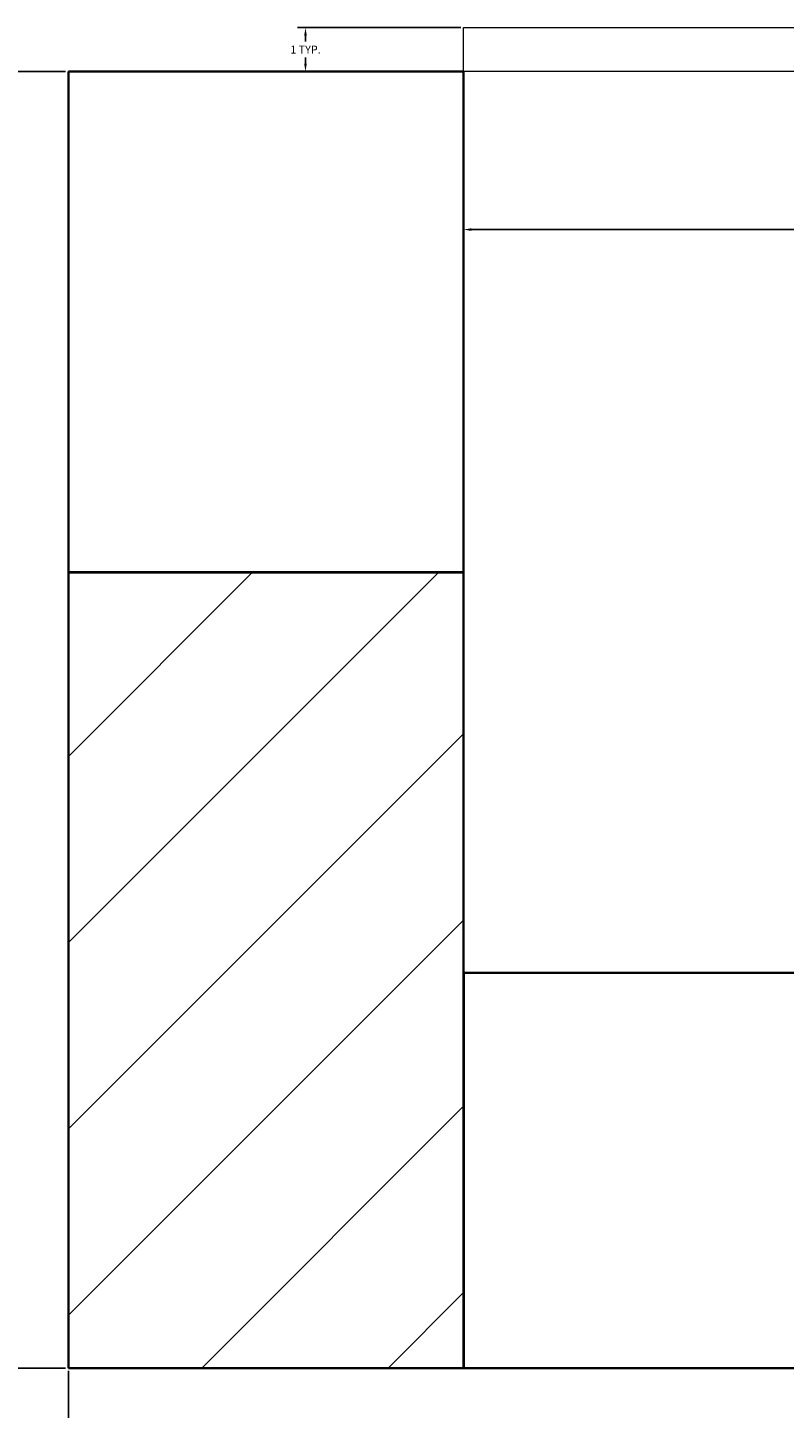
# Model space of a CAD drawing. Units: inches. Extents: x -86 to 2463, y -1058 to 68.
# Tile 5 of 17: x 15 to 32, y -304 to -273. Entities that reach past the tile are written whole.
import ezdxf

# ---------------------------------------------------------------- set-up
doc = ezdxf.new("R2010")
doc.units = ezdxf.units.IN
doc.header["$MEASUREMENT"] = 0
for name, color, linetype, lineweight in [('A-ANNO-DIMS', 2, 'Continuous', 18), ('A-COLS', 7, 'Continuous', 40), ('A-COLS-PATT', 252, 'Continuous', 13), ('A-DOOR', 3, 'Continuous', 18), ('A-WALL', 7, 'Continuous', 35)]:
    doc.layers.add(name, color=color, linetype=linetype, lineweight=lineweight)
doc.styles.get("Standard").update_dxf_attribs({"font": 'arial.ttf'})
doc.dimstyles.get("Standard").update_dxf_attribs({"dimtxt": 0.18, "dimasz": 0.18, "dimexe": 0.18, "dimexo": 0.0625, "dimgap": 0.09, "dimtad": 0, "dimtih": 1, "dimtoh": 1, "dimdec": 4, "dimzin": 0, "dimdsep": 46, "dimtxsty": 'Standard', "dimcen": 0.09, "dimadec": 0, "dimazin": 0, "dimtfac": 1, "dimtdec": 4, "dimtofl": 0, "dimtmove": 0, "dimatfit": 3, "dimfxl": 1, "dimtolj": 1, "dimtzin": 0, "dimarcsym": 0})

# ---------------------------------------------------------------- blocks, each defined once
blk = doc.blocks.new('DOOR-LEAF-24IN')
for p, q in [((0, 0), (0, 24)), ((0, 24), (1, 24)), ((1, 24), (1, 0)), ((1, 0), (0, 0))]:
    blk.add_line(p, q)
blk = doc.blocks.new('*D10')
at = {"layer": 'A-ANNO-DIMS', "color": 0, "lineweight": -2, "transparency": 16777216}
for p, q in [((24.761, -273.637), (24.761, -277.354)), ((48.761, -273.637), (48.761, -277.354)), ((24.941, -277.174), (35.887, -277.174)), ((48.581, -277.174), (37.634, -277.174))]:
    blk.add_line(p, q, dxfattribs=at)
at = {"layer": 'A-ANNO-DIMS', "color": 0, "transparency": 16777216}
for points in [[(24.941, -277.144), (24.941, -277.204), (24.761, -277.174)], [(48.581, -277.144), (48.581, -277.204), (48.761, -277.174)]]:
    blk.add_solid(points, dxfattribs=at)
at = {"layer": 'Defpoints', "color": 0, "transparency": 16777216}
for p in [(24.761, -273.574), (48.761, -273.574), (48.761, -277.174)]:
    blk.add_point(p, dxfattribs=at)
at = {"layer": 'A-ANNO-DIMS', "color": 0, "transparency": 16777216, "insert": (36.761, -277.174), "char_height": 0.18, "attachment_point": 5}
blk.add_mtext('\\A1;LEAF 24 TYP.', dxfattribs=at)
blk = doc.blocks.new('*D11')
at = {"layer": 'A-ANNO-DIMS', "color": 0, "lineweight": -2, "transparency": 16777216}
for p, q in [((24.698, -272.574), (20.981, -272.574)), ((21.161, -272.754), (21.161, -272.894)), ((21.161, -273.394), (21.161, -273.254)), ((24.698, -273.574), (20.981, -273.574))]:
    blk.add_line(p, q, dxfattribs=at)
at = {"layer": 'A-ANNO-DIMS', "color": 0, "transparency": 16777216}
for points in [[(21.131, -272.754), (21.191, -272.754), (21.161, -272.574)], [(21.131, -273.394), (21.191, -273.394), (21.161, -273.574)]]:
    blk.add_solid(points, dxfattribs=at)
at = {"layer": 'Defpoints', "color": 0, "transparency": 16777216}
for p in [(24.761, -272.574), (21.161, -273.574), (24.761, -273.574)]:
    blk.add_point(p, dxfattribs=at)
at = {"layer": 'A-ANNO-DIMS', "color": 0, "transparency": 16777216, "insert": (21.161, -273.074), "char_height": 0.18, "attachment_point": 5}
blk.add_mtext('\\A1;1 TYP.', dxfattribs=at)
blk = doc.blocks.new('*D37')
at = {"layer": 'A-ANNO-DIMS', "color": 0, "lineweight": -2, "transparency": 16777216}
for p, q in [((15.698, -273.574), (-86.019, -273.574)), ((-85.839, -273.754), (-85.839, -288.157)), ((-85.839, -302.924), (-85.839, -288.521)), ((15.698, -303.104), (-86.019, -303.104))]:
    blk.add_line(p, q, dxfattribs=at)
at = {"layer": 'A-ANNO-DIMS', "color": 0, "transparency": 16777216}
for points in [[(-85.869, -273.754), (-85.809, -273.754), (-85.839, -273.574)], [(-85.869, -302.924), (-85.809, -302.924), (-85.839, -303.104)]]:
    blk.add_solid(points, dxfattribs=at)
at = {"layer": 'Defpoints', "color": 0, "transparency": 16777216}
for p in [(-85.839, -273.574), (15.761, -273.574), (15.761, -303.104)]:
    blk.add_point(p, dxfattribs=at)
at = {"layer": 'A-ANNO-DIMS', "color": 0, "transparency": 16777216, "insert": (-85.839, -288.339), "char_height": 0.18, "attachment_point": 5}
blk.add_mtext('\\A1;29.53', dxfattribs=at)
blk = doc.blocks.new('*D38')
at = {"layer": 'A-ANNO-DIMS', "color": 0, "lineweight": -2, "transparency": 16777216}
for p, q in [((15.698, -222.104), (-86.019, -222.104)), ((-85.839, -222.284), (-85.839, -247.657)), ((-85.839, -273.394), (-85.839, -248.021)), ((15.698, -273.574), (-86.019, -273.574))]:
    blk.add_line(p, q, dxfattribs=at)
at = {"layer": 'A-ANNO-DIMS', "color": 0, "transparency": 16777216}
for points in [[(-85.869, -222.284), (-85.809, -222.284), (-85.839, -222.104)], [(-85.869, -273.394), (-85.809, -273.394), (-85.839, -273.574)]]:
    blk.add_solid(points, dxfattribs=at)
at = {"layer": 'Defpoints', "color": 0, "transparency": 16777216}
for p in [(-85.839, -222.104), (15.761, -222.104), (15.761, -273.574)]:
    blk.add_point(p, dxfattribs=at)
at = {"layer": 'A-ANNO-DIMS', "color": 0, "transparency": 16777216, "insert": (-85.839, -247.839), "char_height": 0.18, "attachment_point": 5}
blk.add_mtext('\\A1;51.47', dxfattribs=at)
blk = doc.blocks.new('*D41')
at = {"layer": 'A-ANNO-DIMS', "color": 0, "lineweight": -2, "transparency": 16777216}
for p, q in [((15.761, -303.167), (15.761, -740.384)), ((68.889, -303.167), (68.889, -740.384)), ((15.941, -740.204), (41.931, -740.204)), ((68.709, -740.204), (42.719, -740.204))]:
    blk.add_line(p, q, dxfattribs=at)
at = {"layer": 'A-ANNO-DIMS', "color": 0, "transparency": 16777216}
for points in [[(15.941, -740.174), (15.941, -740.234), (15.761, -740.204)], [(68.709, -740.174), (68.709, -740.234), (68.889, -740.204)]]:
    blk.add_solid(points, dxfattribs=at)
at = {"layer": 'Defpoints', "color": 0, "transparency": 16777216}
for p in [(15.761, -303.104), (68.889, -303.104), (68.889, -740.204)]:
    blk.add_point(p, dxfattribs=at)
at = {"layer": 'A-ANNO-DIMS', "color": 0, "transparency": 16777216, "insert": (42.325, -740.204), "char_height": 0.18, "attachment_point": 5}
blk.add_mtext('\\A1;53.13', dxfattribs=at)

msp = doc.modelspace()

# ---------------------------------------------------------------- hatches: boundary and pattern name
at = {"layer": 'A-COLS-PATT'}
h = msp.add_hatch(dxfattribs=at)
h.set_pattern_fill('ANSI31', color=256, scale=24)
h.set_pattern_definition([(45, (-1015.1314, -586.0864), (-2.1213203, 2.1213203), [])])
h.paths.add_polyline_path([(24.761, -294.104), (24.761, -284.978), (15.761, -284.978), (15.761, -303.104), (24.761, -303.104)])
h.paths.add_polyline_path([(199.1, -294.104), (183.761, -294.104), (183.761, -303.104), (199.1, -303.104)])
h.paths.add_polyline_path([(386.761, -294.104), (377.761, -294.104), (369.914, -294.104), (369.914, -303.104), (377.846, -303.104), (386.761, -303.104)])
h.paths.add_polyline_path([(386.761, -145.104), (386.761, -141.104), (377.761, -141.104), (377.761, -145.104), (377.761, -154.61), (386.761, -154.61)])
h.paths.add_polyline_path([(386.761, -154.61), (377.761, -154.61), (377.761, -162.891), (386.761, -162.891)])
h.paths.add_polyline_path([(24.761, -145.104), (24.761, -141.104), (15.761, -141.104), (15.761, -156.678), (24.761, -156.678)])
h.paths.add_polyline_path([(-38.239, 28.896), (-47.239, 28.896), (-47.239, 19.896), (-47.239, 12.652), (-38.239, 12.652), (-38.239, 19.896)])
h.paths.add_polyline_path([(24.761, 28.896), (15.761, 28.896), (15.761, 19.896), (15.761, 12.545), (24.761, 12.545), (24.761, 19.896)])
h.paths.add_polyline_path([(183.507, 19.896), (161.036, 19.896), (161.036, 17.001), (183.507, 17.001)])
h.paths.add_polyline_path([(183.507, 28.896), (161.036, 28.896), (161.036, 19.896), (183.507, 19.896)])
h.paths.add_polyline_path([(386.761, 28.896), (373.166, 28.896), (373.166, 19.896), (377.761, 19.896), (386.761, 19.896)])

# ---------------------------------------------------------------- linework, layer by layer
at = {"layer": 'A-COLS'}
for p, q in [((15.761, -284.978), (24.761, -284.978)), ((24.761, -294.104), (24.761, -303.104))]:
    msp.add_line(p, q, dxfattribs=at)
at = {"layer": 'A-WALL'}
for p, q in [((15.761, -273.574), (24.761, -273.574)), ((15.761, -273.574), (15.761, -303.104)), ((24.761, -273.574), (24.761, -294.104)), ((183.761, -294.104), (24.761, -294.104)), ((377.846, -303.104), (15.761, -303.104))]:
    msp.add_line(p, q, dxfattribs=at)

# ---------------------------------------------------------------- block references
at = {"layer": 'A-DOOR', "rotation": 270.0000000000001}
msp.add_blockref('DOOR-LEAF-24IN', (24.761, -272.574), dxfattribs=at)

# ---------------------------------------------------------------- dimensions: what is measured, and where the dimension line sits
at = {"layer": 'A-ANNO-DIMS'}
for base, p1, p2, picture, middle in [((-85.839, -222.104), (15.761, -273.574), (15.761, -222.104), '*D38', (-85.839, -247.839)), ((-85.839, -273.574), (15.761, -303.104), (15.761, -273.574), '*D37', (-85.839, -288.339))]:
    dim = msp.add_linear_dim(base=base, p1=p1, p2=p2, angle=90, dimstyle='Standard', override={"dimdec": 2, "dimlfac": 1, "dimrnd": 0, "dimzin": 0, "dimdsep": 46, "dimlunit": 2}, dxfattribs=at)
    dim.commit()
    dim.dimension.update_dxf_attribs({"geometry": picture, "text_midpoint": middle})
dim = msp.add_linear_dim(base=(21.161, -273.574), p1=(24.761, -272.574), p2=(24.761, -273.574), angle=270, text='<> TYP.', dimstyle='Standard', override={"dimdec": 0, "dimlfac": 1, "dimrnd": 0, "dimzin": 0, "dimdsep": 46, "dimlunit": 2}, dxfattribs=at)
dim.commit()
dim.dimension.update_dxf_attribs({"geometry": '*D11', "text_midpoint": (21.161, -273.074)})
dim = msp.add_linear_dim(base=(48.761, -277.174), p1=(24.761, -273.574), p2=(48.761, -273.574), text='LEAF <> TYP.', dimstyle='Standard', override={"dimdec": 0, "dimlfac": 1, "dimrnd": 0, "dimzin": 0, "dimdsep": 46, "dimlunit": 2}, dxfattribs=at)
dim.commit()
dim.dimension.update_dxf_attribs({"geometry": '*D10', "text_midpoint": (36.761, -277.174)})
dim = msp.add_linear_dim(base=(68.889, -740.204), p1=(15.761, -303.104), p2=(68.889, -303.104), dimstyle='Standard', override={"dimdec": 2, "dimlfac": 1, "dimrnd": 0, "dimzin": 0, "dimdsep": 46, "dimlunit": 2}, dxfattribs=at)
dim.commit()
dim.dimension.update_dxf_attribs({"geometry": '*D41', "text_midpoint": (42.325, -740.204)})

doc.saveas('drawing.dxf')
